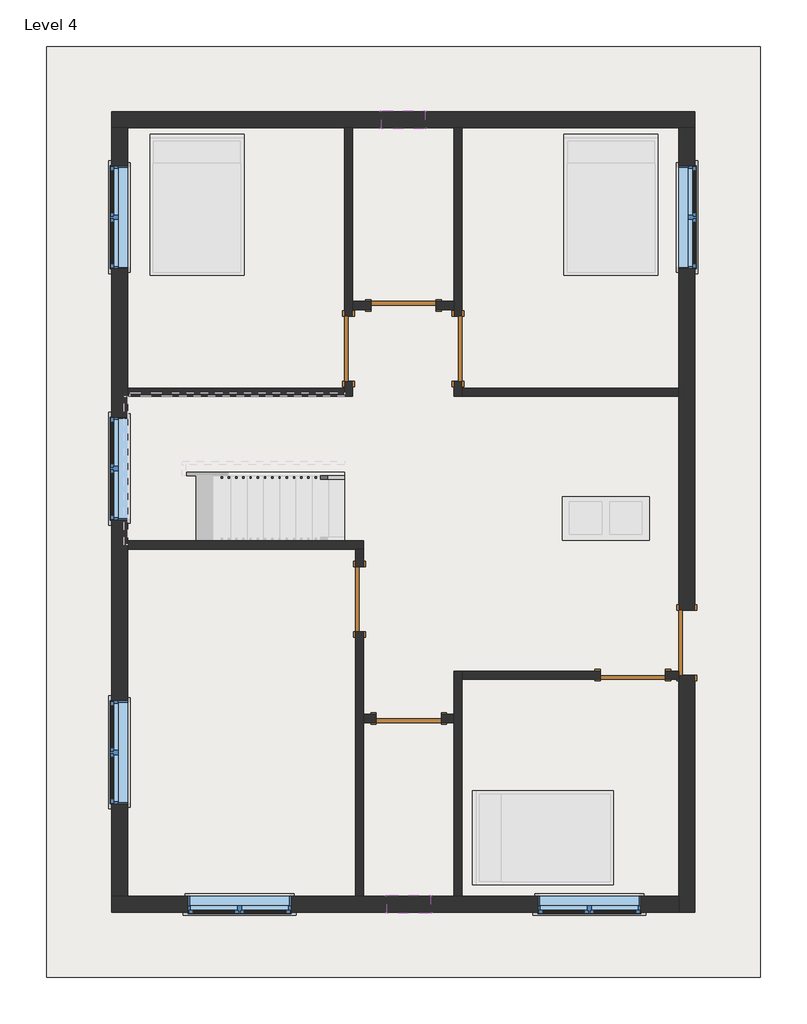
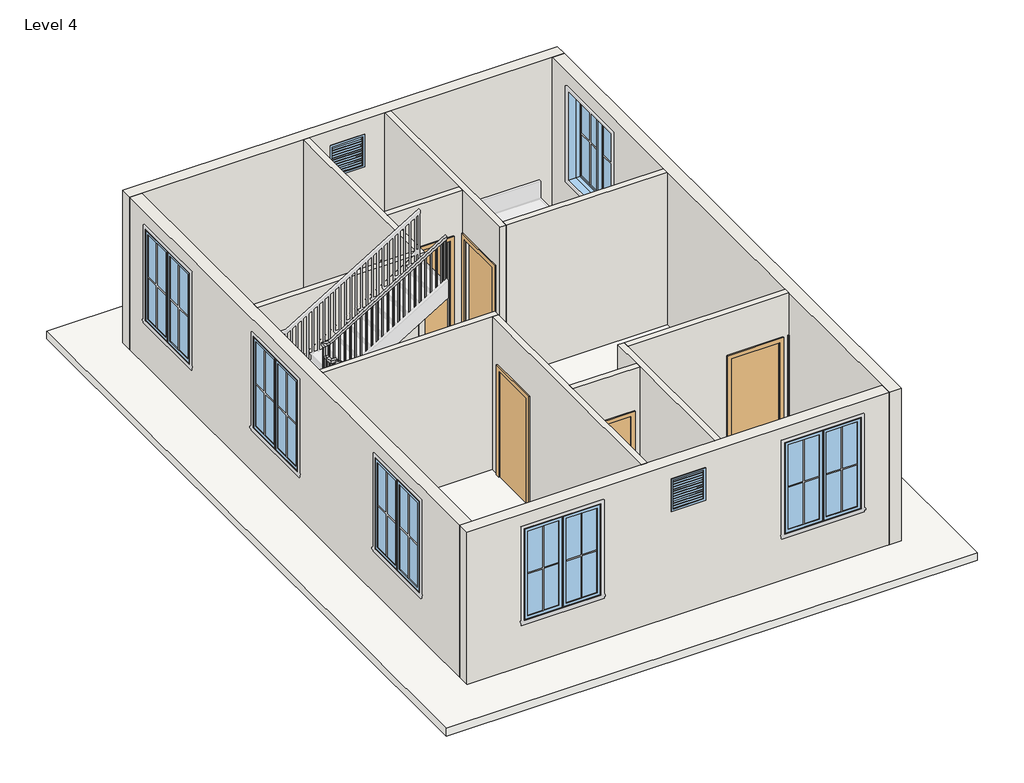
# One storey, part 1 of 2: 14 walls, 8 windows, 7 doors, 1 railing, 1 roof, 1 slab.
"""IFC4 building model written with IfcOpenShell, lengths in millimetres."""

from ifc_helpers import new_model, si_unit, frame, origin, place, context, project, spatial, polyline, outline, extrude, faceted_brep, transform, mapped, element, save
from components import door_305aa2a5, door_e5f9f3c4, door_0ca8825f, window_9ac97e1a, window_f2d8fef0

model = new_model("IFC4")

# Units and contexts
model_context = context("Model", 3, world=origin())
ifc_project = project(units=[si_unit("LENGTHUNIT", "METRE", prefix="MILLI")], contexts=[model_context])

# Site, building, storey
site = spatial("IfcSite", under=ifc_project)
building = spatial("IfcBuilding", under=site)
storey = spatial("IfcBuildingStorey", under=building, Name="Level 4", Elevation=6400.8)

# Doors
placement = place(None, origin())
door_shape = door_305aa2a5(model_context)
element("IfcDoor", 1, ObjectType="Single-Flush : 36\" x 84\"", at=placement, inside=storey, context=model_context, shape_type="MappedRepresentation", body=[
    mapped(door_shape, transform((-2023.6910855, 2116.5303617, 6400.8), x_axis=(0.0, -1.0, 0.0), y_axis=(1.0, 0.0, 0.0), z_axis=(0.0, 0.0, 1.0))),
])
element("IfcDoor", 2, ObjectType="Single-Flush : 36\" x 84\"", at=placement, inside=storey, context=model_context, shape_type="MappedRepresentation", body=[
    mapped(door_shape, transform((-1179.1410855, -3078.1725945, 6400.8), x_axis=(1.0, 0.0, 0.0), y_axis=(0.0, 1.0, 0.0), z_axis=(0.0, 0.0, 1.0))),
])
element("IfcDoor", 3, ObjectType="Single-Flush : 36\" x 84\"", at=placement, inside=storey, context=model_context, shape_type="MappedRepresentation", body=[
    mapped(door_shape, transform((1970.4589145, -2468.1696383, 6400.8), x_axis=(1.0, 0.0, 0.0), y_axis=(0.0, 1.0, 0.0), z_axis=(0.0, 0.0, 1.0))),
])
door_2_shape = door_e5f9f3c4(model_context)
element("IfcDoor", 4, ObjectType="Single-Flush : 36\" x 84\"", at=placement, inside=storey, context=model_context, shape_type="MappedRepresentation", body=[
    mapped(door_2_shape, transform((-486.9910855, 2116.5303617, 6400.8), x_axis=(0.0, -1.0, 0.0), y_axis=(1.0, 0.0, 0.0), z_axis=(0.0, 0.0, 1.0))),
])
element("IfcDoor", 5, ObjectType="Single-Flush : 36\" x 84\"", at=placement, inside=storey, context=model_context, shape_type="MappedRepresentation", body=[
    mapped(door_2_shape, transform((-1871.2910855, -1401.3696383, 6400.8), x_axis=(0.0, 1.0, 0.0), y_axis=(-1.0, 0.0, 0.0), z_axis=(0.0, 0.0, 1.0))),
])
element("IfcDoor", 6, ObjectType="Single-Flush : 36\" x 84\"", at=placement, inside=storey, context=model_context, shape_type="MappedRepresentation", body=[
    mapped(door_2_shape, transform((-1255.3410855, 2726.1303617, 6400.8), x_axis=(1.0, 0.0, 0.0), y_axis=(0.0, 1.0, 0.0), z_axis=(0.0, 0.0, 1.0))),
])
door_3_shape = door_0ca8825f(model_context)
element("IfcDoor", 7, ObjectType="Single-Flush : 36\" x 84\"", at=placement, inside=storey, context=model_context, shape_type="MappedRepresentation", body=[
    mapped(door_3_shape, transform((2732.4589145, -2010.9696383, 6400.8), x_axis=(0.0, 1.0, 0.0), y_axis=(-1.0, 0.0, 0.0), z_axis=(0.0, 0.0, 1.0))),
])

# Railing
element("IfcRailing", 8, ObjectType="Handrail - Rectangular", at=placement, inside=storey, context=model_context, shape_type="SolidModel", body=[
    faceted_brep([(-2080.8410855, 281.3803617, 7453.7454545), (-2080.8410855, 281.3803617, 7394.3439943), (-2080.8410855, 332.1803617, 7394.3439943), (-2080.8410855, 332.1803617, 7453.7454545), (-4290.6410855, 281.3803617, 8793.0181818), (-4341.4410855, 281.3803617, 8764.4046004), (-4341.4410855, 332.1803617, 8764.4046004), (-4290.6410855, 332.1803617, 8793.0181818), (-4290.6410855, 281.3803617, 8839.2), (-4341.4410855, 281.3803617, 8788.4), (-4341.4410855, 332.1803617, 8788.4), (-4290.6410855, 332.1803617, 8839.2), (-4417.6410855, 281.3803617, 8839.2), (-4417.6410855, 281.3803617, 8788.4), (-4366.8410855, 332.1803617, 8788.4), (-4366.8410855, 332.1803617, 8839.2), (-4417.6410855, 408.3803617, 8839.2), (-4417.6410855, 408.3803617, 8788.4), (-4366.8410855, 408.3803617, 8788.4), (-4366.8410855, 408.3803617, 8839.2), (-4417.6410855, 459.1803617, 8839.2), (-4417.6410855, 509.9803617, 8788.4), (-4366.8410855, 509.9803617, 8788.4), (-4366.8410855, 459.1803617, 8839.2), (-4417.6410855, 459.1803617, 9023.9272727), (-4417.6410855, 509.9803617, 8973.1272727), (-4366.8410855, 509.9803617, 8973.1272727), (-4366.8410855, 459.1803617, 9023.9272727), (-4417.6410855, 586.1803617, 9023.9272727), (-4417.6410855, 586.1803617, 8973.1272727), (-4366.8410855, 535.3803617, 8973.1272727), (-4366.8410855, 535.3803617, 9023.9272727), (-4290.6410855, 586.1803617, 9023.9272727), (-4276.4486761, 586.1803617, 8973.1272727), (-4276.4486761, 535.3803617, 8973.1272727), (-4290.6410855, 535.3803617, 9023.9272727), (-2080.8410855, 586.1803617, 10363.2), (-2080.8410855, 535.3803617, 10363.2), (-2080.8410855, 535.3803617, 10303.7985397), (-2080.8410855, 586.1803617, 10303.7985397)], [[[0, 1, 2, 3]], [[1, 0, 4, 5]], [[2, 1, 5, 6]], [[3, 2, 6, 7]], [[0, 3, 7, 4]], [[5, 4, 8, 9]], [[6, 5, 9, 10]], [[7, 6, 10, 11]], [[4, 7, 11, 8]], [[9, 8, 12, 13]], [[10, 9, 13, 14]], [[11, 10, 14, 15]], [[8, 11, 15, 12]], [[13, 12, 16, 17]], [[14, 13, 17, 18]], [[15, 14, 18, 19]], [[12, 15, 19, 16]], [[17, 16, 20, 21]], [[18, 17, 21, 22]], [[19, 18, 22, 23]], [[16, 19, 23, 20]], [[21, 20, 24, 25]], [[22, 21, 25, 26]], [[23, 22, 26, 27]], [[20, 23, 27, 24]], [[25, 24, 28, 29]], [[26, 25, 29, 30]], [[27, 26, 30, 31]], [[24, 27, 31, 28]], [[29, 28, 32, 33]], [[30, 29, 33, 34]], [[31, 30, 34, 35]], [[28, 31, 35, 32]], [[36, 37, 38, 39]], [[33, 32, 36, 39]], [[34, 33, 39, 38]], [[35, 34, 38, 37]], [[32, 35, 37, 36]]]),
    extrude(outline(polyline([(10263.3894488, -2147.5160855), (10251.8439943, -2166.5660855), (9310.2545455, -2166.5660855), (9310.2545455, -2147.5160855), (10263.3894488, -2147.5160855)])), frame((0.0, 551.2553617, 0.0), z_axis=(0.0, 1.0, 0.0), x_axis=(0.0, 0.0, 1.0)), (0.0, 0.0, 1.0), 19.05),
    extrude(outline(polyline([(10201.8136913, -2249.1160855), (10190.2682367, -2268.1660855), (9310.2545455, -2268.1660855), (9310.2545455, -2249.1160855), (10201.8136913, -2249.1160855)])), frame((0.0, 551.2553617, 0.0), z_axis=(0.0, 1.0, 0.0), x_axis=(0.0, 0.0, 1.0)), (0.0, 0.0, 1.0), 19.05),
    extrude(outline(polyline([(10140.2379337, -2350.7160855), (10128.6924791, -2369.7660855), (9171.7090909, -2369.7660855), (9171.7090909, -2350.7160855), (10140.2379337, -2350.7160855)])), frame((0.0, 551.2553617, 0.0), z_axis=(0.0, 1.0, 0.0), x_axis=(0.0, 0.0, 1.0)), (0.0, 0.0, 1.0), 19.05),
    extrude(outline(polyline([(10078.6621761, -2452.3160855), (10067.1167216, -2471.3660855), (9171.7090909, -2471.3660855), (9171.7090909, -2452.3160855), (10078.6621761, -2452.3160855)])), frame((0.0, 551.2553617, 0.0), z_axis=(0.0, 1.0, 0.0), x_axis=(0.0, 0.0, 1.0)), (0.0, 0.0, 1.0), 19.05),
    extrude(outline(polyline([(10017.0864185, -2553.9160855), (10005.540964, -2572.9660855), (9033.1636364, -2572.9660855), (9033.1636364, -2553.9160855), (10017.0864185, -2553.9160855)])), frame((0.0, 551.2553617, 0.0), z_axis=(0.0, 1.0, 0.0), x_axis=(0.0, 0.0, 1.0)), (0.0, 0.0, 1.0), 19.05),
    extrude(outline(polyline([(9955.510661, -2655.5160855), (9943.9652064, -2674.5660855), (9033.1636364, -2674.5660855), (9033.1636364, -2655.5160855), (9955.510661, -2655.5160855)])), frame((0.0, 551.2553617, 0.0), z_axis=(0.0, 1.0, 0.0), x_axis=(0.0, 0.0, 1.0)), (0.0, 0.0, 1.0), 19.05),
    extrude(outline(polyline([(9893.9349034, -2757.1160855), (9882.3894488, -2776.1660855), (9033.1636364, -2776.1660855), (9033.1636364, -2757.1160855), (9893.9349034, -2757.1160855)])), frame((0.0, 551.2553617, 0.0), z_axis=(0.0, 1.0, 0.0), x_axis=(0.0, 0.0, 1.0)), (0.0, 0.0, 1.0), 19.05),
    extrude(outline(polyline([(9832.3591458, -2858.7160855), (9820.8136913, -2877.7660855), (8894.6181818, -2877.7660855), (8894.6181818, -2858.7160855), (9832.3591458, -2858.7160855)])), frame((0.0, 551.2553617, 0.0), z_axis=(0.0, 1.0, 0.0), x_axis=(0.0, 0.0, 1.0)), (0.0, 0.0, 1.0), 19.05),
    extrude(outline(polyline([(9770.7833882, -2960.3160855), (9759.2379337, -2979.3660855), (8894.6181818, -2979.3660855), (8894.6181818, -2960.3160855), (9770.7833882, -2960.3160855)])), frame((0.0, 551.2553617, 0.0), z_axis=(0.0, 1.0, 0.0), x_axis=(0.0, 0.0, 1.0)), (0.0, 0.0, 1.0), 19.05),
    extrude(outline(polyline([(9709.2076307, -3061.9160855), (9697.6621761, -3080.9660855), (8756.0727273, -3080.9660855), (8756.0727273, -3061.9160855), (9709.2076307, -3061.9160855)])), frame((0.0, 551.2553617, 0.0), z_axis=(0.0, 1.0, 0.0), x_axis=(0.0, 0.0, 1.0)), (0.0, 0.0, 1.0), 19.05),
    extrude(outline(polyline([(9647.6318731, -3163.5160855), (9636.0864185, -3182.5660855), (8756.0727273, -3182.5660855), (8756.0727273, -3163.5160855), (9647.6318731, -3163.5160855)])), frame((0.0, 551.2553617, 0.0), z_axis=(0.0, 1.0, 0.0), x_axis=(0.0, 0.0, 1.0)), (0.0, 0.0, 1.0), 19.05),
    extrude(outline(polyline([(9586.0561155, -3265.1160855), (9574.510661, -3284.1660855), (8617.5272727, -3284.1660855), (8617.5272727, -3265.1160855), (9586.0561155, -3265.1160855)])), frame((0.0, 551.2553617, 0.0), z_axis=(0.0, 1.0, 0.0), x_axis=(0.0, 0.0, 1.0)), (0.0, 0.0, 1.0), 19.05),
    extrude(outline(polyline([(9524.4803579, -3366.7160855), (9512.9349034, -3385.7660855), (8617.5272727, -3385.7660855), (8617.5272727, -3366.7160855), (9524.4803579, -3366.7160855)])), frame((0.0, 551.2553617, 0.0), z_axis=(0.0, 1.0, 0.0), x_axis=(0.0, 0.0, 1.0)), (0.0, 0.0, 1.0), 19.05),
    extrude(outline(polyline([(9462.9046004, -3468.3160855), (9451.3591458, -3487.3660855), (8478.9818182, -3487.3660855), (8478.9818182, -3468.3160855), (9462.9046004, -3468.3160855)])), frame((0.0, 551.2553617, 0.0), z_axis=(0.0, 1.0, 0.0), x_axis=(0.0, 0.0, 1.0)), (0.0, 0.0, 1.0), 19.05),
    extrude(outline(polyline([(9401.3288428, -3569.9160855), (9389.7833882, -3588.9660855), (8478.9818182, -3588.9660855), (8478.9818182, -3569.9160855), (9401.3288428, -3569.9160855)])), frame((0.0, 551.2553617, 0.0), z_axis=(0.0, 1.0, 0.0), x_axis=(0.0, 0.0, 1.0)), (0.0, 0.0, 1.0), 19.05),
    extrude(outline(polyline([(9339.7530852, -3671.5160855), (9328.2076307, -3690.5660855), (8478.9818182, -3690.5660855), (8478.9818182, -3671.5160855), (9339.7530852, -3671.5160855)])), frame((0.0, 551.2553617, 0.0), z_axis=(0.0, 1.0, 0.0), x_axis=(0.0, 0.0, 1.0)), (0.0, 0.0, 1.0), 19.05),
    extrude(outline(polyline([(9278.1773276, -3773.1160855), (9266.6318731, -3792.1660855), (8340.4363636, -3792.1660855), (8340.4363636, -3773.1160855), (9278.1773276, -3773.1160855)])), frame((0.0, 551.2553617, 0.0), z_axis=(0.0, 1.0, 0.0), x_axis=(0.0, 0.0, 1.0)), (0.0, 0.0, 1.0), 19.05),
    extrude(outline(polyline([(9216.60157, -3874.7160855), (9205.0561155, -3893.7660855), (8340.4363636, -3893.7660855), (8340.4363636, -3874.7160855), (9216.60157, -3874.7160855)])), frame((0.0, 551.2553617, 0.0), z_axis=(0.0, 1.0, 0.0), x_axis=(0.0, 0.0, 1.0)), (0.0, 0.0, 1.0), 19.05),
    extrude(outline(polyline([(9155.0258125, -3976.3160855), (9143.4803579, -3995.3660855), (8201.8909091, -3995.3660855), (8201.8909091, -3976.3160855), (9155.0258125, -3976.3160855)])), frame((0.0, 551.2553617, 0.0), z_axis=(0.0, 1.0, 0.0), x_axis=(0.0, 0.0, 1.0)), (0.0, 0.0, 1.0), 19.05),
    extrude(outline(polyline([(9093.4500549, -4077.9160855), (9081.9046004, -4096.9660855), (8201.8909091, -4096.9660855), (8201.8909091, -4077.9160855), (9093.4500549, -4077.9160855)])), frame((0.0, 551.2553617, 0.0), z_axis=(0.0, 1.0, 0.0), x_axis=(0.0, 0.0, 1.0)), (0.0, 0.0, 1.0), 19.05),
    extrude(outline(polyline([(9031.8742973, -4179.5160855), (9020.3288428, -4198.5660855), (8063.3454545, -4198.5660855), (8063.3454545, -4179.5160855), (9031.8742973, -4179.5160855)])), frame((0.0, 551.2553617, 0.0), z_axis=(0.0, 1.0, 0.0), x_axis=(0.0, 0.0, 1.0)), (0.0, 0.0, 1.0), 19.05),
    extrude(outline(polyline([(8970.2985397, -4281.1160855), (8958.7530852, -4300.1660855), (8063.3454545, -4300.1660855), (8063.3454545, -4281.1160855), (8970.2985397, -4281.1160855)])), frame((0.0, 551.2553617, 0.0), z_axis=(0.0, 1.0, 0.0), x_axis=(0.0, 0.0, 1.0)), (0.0, 0.0, 1.0), 19.05),
    extrude(outline(polyline([(-4382.7160855, 500.4553617), (-4401.7660855, 500.4553617), (-4401.7660855, 519.5053617), (-4382.7160855, 519.5053617), (-4382.7160855, 500.4553617)])), frame((0.0, 0.0, 7924.8), z_axis=(0.0, 0.0, 1.0), x_axis=(1.0, 0.0, 0.0)), (0.0, 0.0, 1.0), 1048.3272727),
    extrude(outline(polyline([(-4382.7160855, 398.8553617), (-4401.7660855, 398.8553617), (-4401.7660855, 417.9053617), (-4382.7160855, 417.9053617), (-4382.7160855, 398.8553617)])), frame((0.0, 0.0, 7924.8), z_axis=(0.0, 0.0, 1.0), x_axis=(1.0, 0.0, 0.0)), (0.0, 0.0, 1.0), 863.6),
    extrude(outline(polyline([(-4306.5160855, 316.3053617), (-4306.5160855, 297.2553617), (-4325.5660855, 297.2553617), (-4325.5660855, 316.3053617), (-4306.5160855, 316.3053617)])), frame((0.0, 0.0, 7786.2545455), z_axis=(0.0, 0.0, 1.0), x_axis=(1.0, 0.0, 0.0)), (0.0, 0.0, 1.0), 1002.1454545),
    extrude(outline(polyline([(8681.6621761, -4204.9160855), (8693.2076307, -4223.9660855), (7786.2545455, -4223.9660855), (7786.2545455, -4204.9160855), (8681.6621761, -4204.9160855)])), frame((0.0, 297.2553617, 0.0), z_axis=(0.0, 1.0, 0.0), x_axis=(0.0, 0.0, 1.0)), (0.0, 0.0, 1.0), 19.05),
    extrude(outline(polyline([(8620.0864185, -4103.3160855), (8631.6318731, -4122.3660855), (7647.7090909, -4122.3660855), (7647.7090909, -4103.3160855), (8620.0864185, -4103.3160855)])), frame((0.0, 297.2553617, 0.0), z_axis=(0.0, 1.0, 0.0), x_axis=(0.0, 0.0, 1.0)), (0.0, 0.0, 1.0), 19.05),
    extrude(outline(polyline([(8558.510661, -4001.7160855), (8570.0561155, -4020.7660855), (7647.7090909, -4020.7660855), (7647.7090909, -4001.7160855), (8558.510661, -4001.7160855)])), frame((0.0, 297.2553617, 0.0), z_axis=(0.0, 1.0, 0.0), x_axis=(0.0, 0.0, 1.0)), (0.0, 0.0, 1.0), 19.05),
    extrude(outline(polyline([(8496.9349034, -3900.1160855), (8508.4803579, -3919.1660855), (7647.7090909, -3919.1660855), (7647.7090909, -3900.1160855), (8496.9349034, -3900.1160855)])), frame((0.0, 297.2553617, 0.0), z_axis=(0.0, 1.0, 0.0), x_axis=(0.0, 0.0, 1.0)), (0.0, 0.0, 1.0), 19.05),
    extrude(outline(polyline([(8435.3591458, -3798.5160855), (8446.9046004, -3817.5660855), (7509.1636364, -3817.5660855), (7509.1636364, -3798.5160855), (8435.3591458, -3798.5160855)])), frame((0.0, 297.2553617, 0.0), z_axis=(0.0, 1.0, 0.0), x_axis=(0.0, 0.0, 1.0)), (0.0, 0.0, 1.0), 19.05),
    extrude(outline(polyline([(8373.7833882, -3696.9160855), (8385.3288428, -3715.9660855), (7509.1636364, -3715.9660855), (7509.1636364, -3696.9160855), (8373.7833882, -3696.9160855)])), frame((0.0, 297.2553617, 0.0), z_axis=(0.0, 1.0, 0.0), x_axis=(0.0, 0.0, 1.0)), (0.0, 0.0, 1.0), 19.05),
    extrude(outline(polyline([(8312.2076307, -3595.3160855), (8323.7530852, -3614.3660855), (7370.6181818, -3614.3660855), (7370.6181818, -3595.3160855), (8312.2076307, -3595.3160855)])), frame((0.0, 297.2553617, 0.0), z_axis=(0.0, 1.0, 0.0), x_axis=(0.0, 0.0, 1.0)), (0.0, 0.0, 1.0), 19.05),
    extrude(outline(polyline([(8250.6318731, -3493.7160855), (8262.1773276, -3512.7660855), (7370.6181818, -3512.7660855), (7370.6181818, -3493.7160855), (8250.6318731, -3493.7160855)])), frame((0.0, 297.2553617, 0.0), z_axis=(0.0, 1.0, 0.0), x_axis=(0.0, 0.0, 1.0)), (0.0, 0.0, 1.0), 19.05),
    extrude(outline(polyline([(8189.0561155, -3392.1160855), (8200.60157, -3411.1660855), (7232.0727273, -3411.1660855), (7232.0727273, -3392.1160855), (8189.0561155, -3392.1160855)])), frame((0.0, 297.2553617, 0.0), z_axis=(0.0, 1.0, 0.0), x_axis=(0.0, 0.0, 1.0)), (0.0, 0.0, 1.0), 19.05),
    extrude(outline(polyline([(8127.4803579, -3290.5160855), (8139.0258125, -3309.5660855), (7232.0727273, -3309.5660855), (7232.0727273, -3290.5160855), (8127.4803579, -3290.5160855)])), frame((0.0, 297.2553617, 0.0), z_axis=(0.0, 1.0, 0.0), x_axis=(0.0, 0.0, 1.0)), (0.0, 0.0, 1.0), 19.05),
    extrude(outline(polyline([(8065.9046004, -3188.9160855), (8077.4500549, -3207.9660855), (7093.5272727, -3207.9660855), (7093.5272727, -3188.9160855), (8065.9046004, -3188.9160855)])), frame((0.0, 297.2553617, 0.0), z_axis=(0.0, 1.0, 0.0), x_axis=(0.0, 0.0, 1.0)), (0.0, 0.0, 1.0), 19.05),
    extrude(outline(polyline([(8004.3288428, -3087.3160855), (8015.8742973, -3106.3660855), (7093.5272727, -3106.3660855), (7093.5272727, -3087.3160855), (8004.3288428, -3087.3160855)])), frame((0.0, 297.2553617, 0.0), z_axis=(0.0, 1.0, 0.0), x_axis=(0.0, 0.0, 1.0)), (0.0, 0.0, 1.0), 19.05),
    extrude(outline(polyline([(7942.7530852, -2985.7160855), (7954.2985397, -3004.7660855), (7093.5272727, -3004.7660855), (7093.5272727, -2985.7160855), (7942.7530852, -2985.7160855)])), frame((0.0, 297.2553617, 0.0), z_axis=(0.0, 1.0, 0.0), x_axis=(0.0, 0.0, 1.0)), (0.0, 0.0, 1.0), 19.05),
    extrude(outline(polyline([(7881.1773276, -2884.1160855), (7892.7227822, -2903.1660855), (6954.9818182, -2903.1660855), (6954.9818182, -2884.1160855), (7881.1773276, -2884.1160855)])), frame((0.0, 297.2553617, 0.0), z_axis=(0.0, 1.0, 0.0), x_axis=(0.0, 0.0, 1.0)), (0.0, 0.0, 1.0), 19.05),
    extrude(outline(polyline([(7819.60157, -2782.5160855), (7831.1470246, -2801.5660855), (6954.9818182, -2801.5660855), (6954.9818182, -2782.5160855), (7819.60157, -2782.5160855)])), frame((0.0, 297.2553617, 0.0), z_axis=(0.0, 1.0, 0.0), x_axis=(0.0, 0.0, 1.0)), (0.0, 0.0, 1.0), 19.05),
    extrude(outline(polyline([(7758.0258125, -2680.9160855), (7769.571267, -2699.9660855), (6816.4363636, -2699.9660855), (6816.4363636, -2680.9160855), (7758.0258125, -2680.9160855)])), frame((0.0, 297.2553617, 0.0), z_axis=(0.0, 1.0, 0.0), x_axis=(0.0, 0.0, 1.0)), (0.0, 0.0, 1.0), 19.05),
    extrude(outline(polyline([(7696.4500549, -2579.3160855), (7707.9955094, -2598.3660855), (6816.4363636, -2598.3660855), (6816.4363636, -2579.3160855), (7696.4500549, -2579.3160855)])), frame((0.0, 297.2553617, 0.0), z_axis=(0.0, 1.0, 0.0), x_axis=(0.0, 0.0, 1.0)), (0.0, 0.0, 1.0), 19.05),
    extrude(outline(polyline([(7634.8742973, -2477.7160855), (7646.4197519, -2496.7660855), (6677.8909091, -2496.7660855), (6677.8909091, -2477.7160855), (7634.8742973, -2477.7160855)])), frame((0.0, 297.2553617, 0.0), z_axis=(0.0, 1.0, 0.0), x_axis=(0.0, 0.0, 1.0)), (0.0, 0.0, 1.0), 19.05),
    extrude(outline(polyline([(7573.2985397, -2376.1160855), (7584.8439943, -2395.1660855), (6677.8909091, -2395.1660855), (6677.8909091, -2376.1160855), (7573.2985397, -2376.1160855)])), frame((0.0, 297.2553617, 0.0), z_axis=(0.0, 1.0, 0.0), x_axis=(0.0, 0.0, 1.0)), (0.0, 0.0, 1.0), 19.05),
    extrude(outline(polyline([(7511.7227822, -2274.5160855), (7523.2682367, -2293.5660855), (6539.3454545, -2293.5660855), (6539.3454545, -2274.5160855), (7511.7227822, -2274.5160855)])), frame((0.0, 297.2553617, 0.0), z_axis=(0.0, 1.0, 0.0), x_axis=(0.0, 0.0, 1.0)), (0.0, 0.0, 1.0), 19.05),
    extrude(outline(polyline([(7450.1470246, -2172.9160855), (7461.6924791, -2191.9660855), (6539.3454545, -2191.9660855), (6539.3454545, -2172.9160855), (7450.1470246, -2172.9160855)])), frame((0.0, 297.2553617, 0.0), z_axis=(0.0, 1.0, 0.0), x_axis=(0.0, 0.0, 1.0)), (0.0, 0.0, 1.0), 19.05),
    extrude(outline(polyline([(-4382.7160855, 551.2553617), (-4401.7660855, 551.2553617), (-4401.7660855, 570.3053617), (-4382.7160855, 570.3053617), (-4382.7160855, 551.2553617)])), frame((0.0, 0.0, 7924.8), z_axis=(0.0, 0.0, 1.0), x_axis=(1.0, 0.0, 0.0)), (0.0, 0.0, 1.0), 1048.3272727),
    extrude(outline(polyline([(-4382.7160855, 316.3053617), (-4382.7160855, 297.2553617), (-4401.7660855, 297.2553617), (-4401.7660855, 316.3053617), (-4382.7160855, 316.3053617)])), frame((0.0, 0.0, 7924.8), z_axis=(0.0, 0.0, 1.0), x_axis=(1.0, 0.0, 0.0)), (0.0, 0.0, 1.0), 863.6),
    extrude(outline(polyline([(10303.7985397, -2080.8410855), (10292.2530852, -2099.8910855), (9310.2545455, -2099.8910855), (9310.2545455, -2080.8410855), (10303.7985397, -2080.8410855)])), frame((0.0, 551.2553617, 0.0), z_axis=(0.0, 1.0, 0.0), x_axis=(0.0, 0.0, 1.0)), (0.0, 0.0, 1.0), 19.05),
    extrude(outline(polyline([(7394.3439943, -2080.8410855), (7405.8894488, -2099.8910855), (6539.3454545, -2099.8910855), (6539.3454545, -2080.8410855), (7394.3439943, -2080.8410855)])), frame((0.0, 297.2553617, 0.0), z_axis=(0.0, 1.0, 0.0), x_axis=(0.0, 0.0, 1.0)), (0.0, 0.0, 1.0), 19.05),
])

# Roof
element("IfcRoof", 9, ObjectType="ROOF 6\"", at=placement, inside=storey, context=model_context, shape_type="SweptSolid", body=[
    extrude(outline(polyline([(-6271.8410855, 6364.6803617), (3761.1589145, 6364.6803617), (3761.1589145, -6716.3196383), (-6271.8410855, -6716.3196383), (-6271.8410855, 6364.6803617)])), frame((0.0, 0.0, 6248.4), z_axis=(0.0, 0.0, 1.0), x_axis=(1.0, 0.0, 0.0)), (0.0, 0.0, 1.0), 152.4),
])

# Slab
element("IfcSlab", 10, ObjectType="FLOOR 6\"", at=placement, inside=storey, context=model_context, shape_type="SweptSolid", body=[
    extrude(outline(polyline([(2846.7589145, 5450.2803617), (2846.7589145, -5801.9196383), (-5357.4410855, -5801.9196383), (-5357.4410855, 5450.2803617), (2846.7589145, 5450.2803617)])), frame((0.0, 0.0, 6248.4), z_axis=(0.0, 0.0, 1.0), x_axis=(1.0, 0.0, 0.0)), (0.0, 0.0, 1.0), 152.4),
])

# Walls
element("IfcWall", 11, ObjectType="WALL 4.5\"", at=placement, inside=storey, context=model_context, shape_type="Brep", body=[
    faceted_brep([(-2080.8410855, 1659.3303617, 8534.4), (-2080.8410855, 1659.3303617, 6400.8), (-2080.8410855, 1564.0803617, 6400.8), (-2080.8410855, 1449.7803617, 6400.8), (-2080.8410855, 1449.7803617, 9448.8), (-2080.8410855, 1564.0803617, 9448.8), (-2080.8410855, 5221.6803617, 9448.8), (-2080.8410855, 5221.6803617, 6400.8), (-2080.8410855, 2573.7303617, 6400.8), (-2080.8410855, 2573.7303617, 8534.4), (-1966.5410855, 1449.7803617, 6400.8), (-1966.5410855, 1659.3303617, 6400.8), (-1966.5410855, 1659.3303617, 8534.4), (-1966.5410855, 2573.7303617, 8534.4), (-1966.5410855, 2573.7303617, 6400.8), (-1966.5410855, 2668.9803617, 6400.8), (-1966.5410855, 2783.2803617, 6400.8), (-1966.5410855, 5221.6803617, 6400.8), (-1966.5410855, 5221.6803617, 9448.8), (-1966.5410855, 2783.2803617, 9448.8), (-1966.5410855, 2668.9803617, 9448.8), (-1966.5410855, 1449.7803617, 9448.8)], [[[0, 1, 2, 3, 4, 5, 6, 7, 8, 9]], [[10, 11, 12, 13, 14, 15, 16, 17, 18, 19, 20, 21]], [[8, 7, 17, 16, 15, 14]], [[3, 2, 1, 11, 10]], [[7, 6, 18, 17]], [[4, 3, 10, 21]], [[12, 11, 1, 0]], [[13, 12, 0, 9]], [[14, 13, 9, 8]], [[6, 5, 4, 21, 20, 19, 18]]]),
])
element("IfcWall", 12, ObjectType="WALL 4.5\"", at=placement, inside=storey, context=model_context, shape_type="SweptSolid", body=[
    extrude(outline(polyline([(-5128.8410855, 1564.0803617), (-2080.8410855, 1564.0803617), (-2080.8410855, 1449.7803617), (-5128.8410855, 1449.7803617), (-5128.8410855, 1564.0803617)])), frame((0.0, 0.0, 6400.8), z_axis=(0.0, 0.0, 1.0), x_axis=(1.0, 0.0, 0.0)), (0.0, 0.0, 1.0), 3048.0),
])
element("IfcWall", 13, ObjectType="WALL 4.5\"", at=placement, inside=storey, context=model_context, shape_type="Brep", body=[
    faceted_brep([(-544.1410855, 1659.3303617, 8534.4), (-544.1410855, 1659.3303617, 6400.8), (-544.1410855, 1449.7803617, 6400.8), (-544.1410855, 1449.7803617, 9448.8), (-544.1410855, 2668.9803617, 9448.8), (-544.1410855, 2783.2803617, 9448.8), (-544.1410855, 5221.6803617, 9448.8), (-544.1410855, 5221.6803617, 6400.8), (-544.1410855, 2783.2803617, 6400.8), (-544.1410855, 2668.9803617, 6400.8), (-544.1410855, 2573.7303617, 6400.8), (-544.1410855, 2573.7303617, 8534.4), (-429.8410855, 1449.7803617, 6400.8), (-429.8410855, 1564.0803617, 6400.8), (-429.8410855, 1659.3303617, 6400.8), (-429.8410855, 1659.3303617, 8534.4), (-429.8410855, 2573.7303617, 8534.4), (-429.8410855, 2573.7303617, 6400.8), (-429.8410855, 5221.6803617, 6400.8), (-429.8410855, 5221.6803617, 9448.8), (-429.8410855, 1564.0803617, 9448.8), (-429.8410855, 1449.7803617, 9448.8)], [[[0, 1, 2, 3, 4, 5, 6, 7, 8, 9, 10, 11]], [[12, 13, 14, 15, 16, 17, 18, 19, 20, 21]], [[2, 1, 14, 13, 12]], [[10, 9, 8, 7, 18, 17]], [[7, 6, 19, 18]], [[3, 2, 12, 21]], [[15, 14, 1, 0]], [[16, 15, 0, 11]], [[17, 16, 11, 10]], [[6, 5, 4, 3, 21, 20, 19]]]),
])
element("IfcWall", 14, ObjectType="WALL 4.5\"", at=placement, inside=storey, context=model_context, shape_type="SweptSolid", body=[
    extrude(outline(polyline([(2618.1589145, 1449.7803617), (-429.8410855, 1449.7803617), (-429.8410855, 1564.0803617), (2618.1589145, 1564.0803617), (2618.1589145, 1449.7803617)])), frame((0.0, 0.0, 6400.8), z_axis=(0.0, 0.0, 1.0), x_axis=(1.0, 0.0, 0.0)), (0.0, 0.0, 1.0), 3048.0),
])
element("IfcWall", 15, ObjectType="WALL 4.5\"", at=placement, inside=storey, context=model_context, shape_type="Brep", body=[
    faceted_brep([(-5128.8410855, -696.5196383, 6400.8), (-1928.4410855, -696.5196383, 6400.8), (-1814.1410855, -696.5196383, 6400.8), (-1814.1410855, -696.5196383, 9448.8), (-1928.4410855, -696.5196383, 9448.8), (-5128.8410855, -696.5196383, 9448.8), (-5128.8410855, -582.2196383, 6400.8), (-5128.8410855, -582.2196383, 9448.8), (-1814.1410855, -582.2196383, 9448.8), (-1814.1410855, -582.2196383, 6400.8)], [[[0, 1, 2, 3, 4, 5]], [[6, 7, 8, 9]], [[2, 1, 0, 6, 9]], [[0, 5, 7, 6]], [[3, 2, 9, 8]], [[5, 4, 3, 8, 7]]]),
])
element("IfcWall", 16, ObjectType="WALL 4.5\"", at=placement, inside=storey, context=model_context, shape_type="Brep", body=[
    faceted_brep([(-1814.1410855, -944.1696383, 8534.4), (-1814.1410855, -944.1696383, 6400.8), (-1814.1410855, -696.5196383, 6400.8), (-1814.1410855, -696.5196383, 9448.8), (-1814.1410855, -3021.0225945, 9448.8), (-1814.1410855, -3135.3225945, 9448.8), (-1814.1410855, -5573.3196383, 9448.8), (-1814.1410855, -5573.3196383, 6400.8), (-1814.1410855, -3135.3225945, 6400.8), (-1814.1410855, -3021.0225945, 6400.8), (-1814.1410855, -1858.5696383, 6400.8), (-1814.1410855, -1858.5696383, 8534.4), (-1928.4410855, -696.5196383, 6400.8), (-1928.4410855, -944.1696383, 6400.8), (-1928.4410855, -944.1696383, 8534.4), (-1928.4410855, -1858.5696383, 8534.4), (-1928.4410855, -1858.5696383, 6400.8), (-1928.4410855, -5573.3196383, 6400.8), (-1928.4410855, -5573.3196383, 9448.8), (-1928.4410855, -696.5196383, 9448.8)], [[[0, 1, 2, 3, 4, 5, 6, 7, 8, 9, 10, 11]], [[12, 13, 14, 15, 16, 17, 18, 19]], [[2, 1, 13, 12]], [[10, 9, 8, 7, 17, 16]], [[3, 2, 12, 19]], [[7, 6, 18, 17]], [[14, 13, 1, 0]], [[15, 14, 0, 11]], [[16, 15, 11, 10]], [[6, 5, 4, 3, 19, 18]]]),
])
element("IfcWall", 17, ObjectType="WALL 4.5\"", at=placement, inside=storey, context=model_context, shape_type="SweptSolid", body=[
    extrude(outline(polyline([(8534.4, -721.9410855), (6400.8, -721.9410855), (6400.8, -544.1410855), (9448.8, -544.1410855), (9448.8, -1814.1410855), (6400.8, -1814.1410855), (6400.8, -1636.3410855), (8534.4, -1636.3410855), (8534.4, -721.9410855)])), frame((0.0, -3135.3225945, 0.0), z_axis=(0.0, 1.0, 0.0), x_axis=(0.0, 0.0, 1.0)), (0.0, 0.0, 1.0), 114.3),
])
element("IfcWall", 18, ObjectType="WALL 4.5\"", at=placement, inside=storey, context=model_context, shape_type="Brep", body=[
    faceted_brep([(-544.1410855, -2411.0196383, 6400.8), (-544.1410855, -3021.0225945, 6400.8), (-544.1410855, -3135.3225945, 6400.8), (-544.1410855, -5573.3196383, 6400.8), (-544.1410855, -5573.3196383, 9448.8), (-544.1410855, -3135.3225945, 9448.8), (-544.1410855, -3021.0225945, 9448.8), (-544.1410855, -2411.0196383, 9448.8), (-429.8410855, -2411.0196383, 6400.8), (-429.8410855, -2411.0196383, 9448.8), (-429.8410855, -2525.3196383, 9448.8), (-429.8410855, -5573.3196383, 9448.8), (-429.8410855, -5573.3196383, 6400.8), (-429.8410855, -2525.3196383, 6400.8)], [[[0, 1, 2, 3, 4, 5, 6, 7]], [[8, 9, 10, 11, 12, 13]], [[3, 2, 1, 0, 8, 13, 12]], [[4, 3, 12, 11]], [[0, 7, 9, 8]], [[7, 6, 5, 4, 11, 10, 9]]]),
])
element("IfcWall", 19, ObjectType="WALL 4.5\"", at=placement, inside=storey, context=model_context, shape_type="Brep", body=[
    faceted_brep([(2427.6589145, -2525.3196383, 8534.4), (2427.6589145, -2525.3196383, 6400.8), (2618.1589145, -2525.3196383, 6400.8), (2618.1589145, -2525.3196383, 9448.8), (-429.8410855, -2525.3196383, 9448.8), (-429.8410855, -2525.3196383, 6400.8), (1513.2589145, -2525.3196383, 6400.8), (1513.2589145, -2525.3196383, 8534.4), (2618.1589145, -2411.0196383, 6400.8), (2427.6589145, -2411.0196383, 6400.8), (2427.6589145, -2411.0196383, 8534.4), (1513.2589145, -2411.0196383, 8534.4), (1513.2589145, -2411.0196383, 6400.8), (-429.8410855, -2411.0196383, 6400.8), (-429.8410855, -2411.0196383, 9448.8), (2618.1589145, -2411.0196383, 9448.8), (2618.1589145, -2468.1696383, 6400.8)], [[[0, 1, 2, 3, 4, 5, 6, 7]], [[8, 9, 10, 11, 12, 13, 14, 15]], [[6, 5, 13, 12]], [[2, 1, 9, 8, 16]], [[5, 4, 14, 13]], [[3, 2, 16, 8, 15]], [[10, 9, 1, 0]], [[11, 10, 0, 7]], [[12, 11, 7, 6]], [[4, 3, 15, 14]]]),
])
element("IfcWall", 20, ObjectType="WALL 4.5\"", at=placement, inside=storey, context=model_context, shape_type="SweptSolid", body=[
    extrude(outline(polyline([(8534.4, -798.1410855), (6400.8, -798.1410855), (6400.8, -544.1410855), (9448.8, -544.1410855), (9448.8, -1966.5410855), (6400.8, -1966.5410855), (6400.8, -1712.5410855), (8534.4, -1712.5410855), (8534.4, -798.1410855)])), frame((0.0, 2668.9803617, 0.0), z_axis=(0.0, 1.0, 0.0), x_axis=(0.0, 0.0, 1.0)), (0.0, 0.0, 1.0), 114.3),
])
element("IfcWall", 21, ObjectType="WALL 9\"", at=placement, inside=storey, context=model_context, shape_type="Brep", body=[
    faceted_brep([(-5357.4410855, 5221.6803617, 6400.8), (-5128.8410855, 5221.6803617, 6400.8), (-2080.8410855, 5221.6803617, 6400.8), (-1966.5410855, 5221.6803617, 6400.8), (-544.1410855, 5221.6803617, 6400.8), (-429.8410855, 5221.6803617, 6400.8), (2618.1589145, 5221.6803617, 6400.8), (2846.7589145, 5221.6803617, 6400.8), (2846.7589145, 5221.6803617, 9448.8), (2618.1589145, 5221.6803617, 9448.8), (-429.8410855, 5221.6803617, 9448.8), (-544.1410855, 5221.6803617, 9448.8), (-1966.5410855, 5221.6803617, 9448.8), (-2080.8410855, 5221.6803617, 9448.8), (-5128.8410855, 5221.6803617, 9448.8), (-5357.4410855, 5221.6803617, 9448.8), (-950.5410855, 5221.6803617, 9144.0), (-950.5410855, 5221.6803617, 8534.4), (-1560.1410855, 5221.6803617, 8534.4), (-1560.1410855, 5221.6803617, 9144.0), (-5357.4410855, 5450.2803617, 6400.8), (-5357.4410855, 5450.2803617, 9448.8), (2846.7589145, 5450.2803617, 9448.8), (2846.7589145, 5450.2803617, 6400.8), (-950.5410855, 5450.2803617, 9144.0), (-1560.1410855, 5450.2803617, 9144.0), (-1560.1410855, 5450.2803617, 8534.4), (-950.5410855, 5450.2803617, 8534.4)], [[[0, 1, 2, 3, 4, 5, 6, 7, 8, 9, 10, 11, 12, 13, 14, 15], [16, 17, 18, 19]], [[20, 21, 22, 23], [24, 25, 26, 27]], [[7, 6, 5, 4, 3, 2, 1, 0, 20, 23]], [[8, 7, 23, 22]], [[0, 15, 21, 20]], [[17, 16, 24, 27]], [[18, 17, 27, 26]], [[19, 18, 26, 25]], [[16, 19, 25, 24]], [[15, 14, 13, 12, 11, 10, 9, 8, 22, 21]]]),
])
element("IfcWall", 22, ObjectType="WALL 9\"", at=placement, inside=storey, context=model_context, shape_type="Brep", body=[
    faceted_brep([(2618.1589145, 5221.6803617, 6400.8), (2618.1589145, 1564.0803617, 6400.8), (2618.1589145, 1449.7803617, 6400.8), (2618.1589145, -1553.7696383, 6400.8), (2618.1589145, -1553.7696383, 8534.4), (2618.1589145, -2468.1696383, 8534.4), (2618.1589145, -2468.1696383, 6400.8), (2618.1589145, -2525.3196383, 6400.8), (2618.1589145, -5573.3196383, 6400.8), (2618.1589145, -5801.9196383, 6400.8), (2618.1589145, -5801.9196383, 9448.8), (2618.1589145, -5573.3196383, 9448.8), (2618.1589145, -2525.3196383, 9448.8), (2618.1589145, -2411.0196383, 9448.8), (2618.1589145, 1449.7803617, 9448.8), (2618.1589145, 1564.0803617, 9448.8), (2618.1589145, 5221.6803617, 9448.8), (2618.1589145, 3240.4803617, 9144.0), (2618.1589145, 3240.4803617, 7315.2), (2618.1589145, 4688.2803617, 7315.2), (2618.1589145, 4688.2803617, 9144.0), (2846.7589145, -1553.7696383, 8534.4), (2846.7589145, -1553.7696383, 6400.8), (2846.7589145, 5221.6803617, 6400.8), (2846.7589145, 5221.6803617, 9448.8), (2846.7589145, -5801.9196383, 9448.8), (2846.7589145, -5801.9196383, 6400.8), (2846.7589145, -2468.1696383, 6400.8), (2846.7589145, -2468.1696383, 8534.4), (2846.7589145, 3240.4803617, 9144.0), (2846.7589145, 4688.2803617, 9144.0), (2846.7589145, 4688.2803617, 7315.2), (2846.7589145, 3240.4803617, 7315.2)], [[[0, 1, 2, 3, 4, 5, 6, 7, 8, 9, 10, 11, 12, 13, 14, 15, 16], [17, 18, 19, 20]], [[21, 22, 23, 24, 25, 26, 27, 28], [29, 30, 31, 32]], [[27, 26, 9, 8, 7, 6]], [[23, 22, 3, 2, 1, 0]], [[0, 16, 24, 23]], [[10, 9, 26, 25]], [[18, 17, 29, 32]], [[19, 18, 32, 31]], [[20, 19, 31, 30]], [[17, 20, 30, 29]], [[4, 3, 22, 21]], [[5, 4, 21, 28]], [[6, 5, 28, 27]], [[16, 15, 14, 13, 12, 11, 10, 25, 24]]]),
])
element("IfcWall", 23, ObjectType="WALL 9\"", at=placement, inside=storey, context=model_context, shape_type="Brep", body=[
    faceted_brep([(2618.1589145, -5573.3196383, 6400.8), (-429.8410855, -5573.3196383, 6400.8), (-544.1410855, -5573.3196383, 6400.8), (-1814.1410855, -5573.3196383, 6400.8), (-1928.4410855, -5573.3196383, 6400.8), (-5128.8410855, -5573.3196383, 6400.8), (-5357.4410855, -5573.3196383, 6400.8), (-5357.4410855, -5573.3196383, 9448.8), (-5128.8410855, -5573.3196383, 9448.8), (-1928.4410855, -5573.3196383, 9448.8), (-1814.1410855, -5573.3196383, 9448.8), (-544.1410855, -5573.3196383, 9448.8), (-429.8410855, -5573.3196383, 9448.8), (2618.1589145, -5573.3196383, 9448.8), (-4281.1160855, -5573.3196383, 9144.0), (-4281.1160855, -5573.3196383, 7315.2), (-2833.3160855, -5573.3196383, 7315.2), (-2833.3160855, -5573.3196383, 9144.0), (636.9589145, -5573.3196383, 9144.0), (636.9589145, -5573.3196383, 7315.2), (2084.7589145, -5573.3196383, 7315.2), (2084.7589145, -5573.3196383, 9144.0), (-874.3410855, -5573.3196383, 9144.0), (-1483.9410855, -5573.3196383, 9144.0), (-1483.9410855, -5573.3196383, 8534.4), (-874.3410855, -5573.3196383, 8534.4), (2618.1589145, -5801.9196383, 6400.8), (2618.1589145, -5801.9196383, 9448.8), (-5357.4410855, -5801.9196383, 9448.8), (-5357.4410855, -5801.9196383, 6400.8), (-4281.1160855, -5801.9196383, 9144.0), (-2833.3160855, -5801.9196383, 9144.0), (-2833.3160855, -5801.9196383, 7315.2), (-4281.1160855, -5801.9196383, 7315.2), (636.9589145, -5801.9196383, 9144.0), (2084.7589145, -5801.9196383, 9144.0), (2084.7589145, -5801.9196383, 7315.2), (636.9589145, -5801.9196383, 7315.2), (-874.3410855, -5801.9196383, 9144.0), (-874.3410855, -5801.9196383, 8534.4), (-1483.9410855, -5801.9196383, 8534.4), (-1483.9410855, -5801.9196383, 9144.0)], [[[0, 1, 2, 3, 4, 5, 6, 7, 8, 9, 10, 11, 12, 13], [14, 15, 16, 17], [18, 19, 20, 21], [22, 23, 24, 25]], [[26, 27, 28, 29], [30, 31, 32, 33], [34, 35, 36, 37], [38, 39, 40, 41]], [[6, 5, 4, 3, 2, 1, 0, 26, 29]], [[0, 13, 27, 26]], [[7, 6, 29, 28]], [[15, 14, 30, 33]], [[16, 15, 33, 32]], [[17, 16, 32, 31]], [[14, 17, 31, 30]], [[19, 18, 34, 37]], [[20, 19, 37, 36]], [[21, 20, 36, 35]], [[18, 21, 35, 34]], [[39, 38, 22, 25]], [[40, 39, 25, 24]], [[41, 40, 24, 23]], [[38, 41, 23, 22]], [[13, 12, 11, 10, 9, 8, 7, 28, 27]]]),
])
element("IfcWall", 24, ObjectType="WALL 9\"", at=placement, inside=storey, context=model_context, shape_type="Brep", body=[
    faceted_brep([(-5128.8410855, -5573.3196383, 6400.8), (-5128.8410855, -696.5196383, 6400.8), (-5128.8410855, -582.2196383, 6400.8), (-5128.8410855, 1449.7803617, 6400.8), (-5128.8410855, 1564.0803617, 6400.8), (-5128.8410855, 5221.6803617, 6400.8), (-5128.8410855, 5221.6803617, 9448.8), (-5128.8410855, 1564.0803617, 9448.8), (-5128.8410855, 1449.7803617, 9448.8), (-5128.8410855, -582.2196383, 9448.8), (-5128.8410855, -696.5196383, 9448.8), (-5128.8410855, -5573.3196383, 9448.8), (-5128.8410855, -2830.1196383, 9144.0), (-5128.8410855, -2830.1196383, 7315.2), (-5128.8410855, -4277.9196383, 7315.2), (-5128.8410855, -4277.9196383, 9144.0), (-5128.8410855, 4688.2803617, 9144.0), (-5128.8410855, 4688.2803617, 7315.2), (-5128.8410855, 3240.4803617, 7315.2), (-5128.8410855, 3240.4803617, 9144.0), (-5128.8410855, 1157.6803617, 9144.0), (-5128.8410855, 1157.6803617, 7315.2), (-5128.8410855, -290.1196383, 7315.2), (-5128.8410855, -290.1196383, 9144.0), (-5357.4410855, -5573.3196383, 6400.8), (-5357.4410855, -5573.3196383, 9448.8), (-5357.4410855, 5221.6803617, 9448.8), (-5357.4410855, 5221.6803617, 6400.8), (-5357.4410855, -2830.1196383, 9144.0), (-5357.4410855, -4277.9196383, 9144.0), (-5357.4410855, -4277.9196383, 7315.2), (-5357.4410855, -2830.1196383, 7315.2), (-5357.4410855, 4688.2803617, 9144.0), (-5357.4410855, 3240.4803617, 9144.0), (-5357.4410855, 3240.4803617, 7315.2), (-5357.4410855, 4688.2803617, 7315.2), (-5357.4410855, 1157.6803617, 9144.0), (-5357.4410855, -290.1196383, 9144.0), (-5357.4410855, -290.1196383, 7315.2), (-5357.4410855, 1157.6803617, 7315.2)], [[[0, 1, 2, 3, 4, 5, 6, 7, 8, 9, 10, 11], [12, 13, 14, 15], [16, 17, 18, 19], [20, 21, 22, 23]], [[24, 25, 26, 27], [28, 29, 30, 31], [32, 33, 34, 35], [36, 37, 38, 39]], [[5, 4, 3, 2, 1, 0, 24, 27]], [[6, 5, 27, 26]], [[0, 11, 25, 24]], [[13, 12, 28, 31]], [[14, 13, 31, 30]], [[15, 14, 30, 29]], [[12, 15, 29, 28]], [[17, 16, 32, 35]], [[18, 17, 35, 34]], [[19, 18, 34, 33]], [[16, 19, 33, 32]], [[21, 20, 36, 39]], [[22, 21, 39, 38]], [[23, 22, 38, 37]], [[20, 23, 37, 36]], [[11, 10, 9, 8, 7, 6, 26, 25]]]),
])

# Windows
window_shape = window_9ac97e1a(model_context)
element("IfcWindow", 25, ObjectType="Window-Casement-Double : 57\" x 72\"", at=placement, inside=storey, context=model_context, shape_type="MappedRepresentation", body=[
    mapped(window_shape, transform((-3557.2160855, -5687.6196383, 6400.8), x_axis=(-1.0, 0.0, 0.0), y_axis=(0.0, -1.0, 0.0), z_axis=(0.0, 0.0, 1.0))),
])
element("IfcWindow", 26, ObjectType="Window-Casement-Double : 57\" x 72\"", at=placement, inside=storey, context=model_context, shape_type="MappedRepresentation", body=[
    mapped(window_shape, transform((-5243.1410855, -3554.0196383, 6400.8), x_axis=(0.0, 1.0, 0.0), y_axis=(-1.0, 0.0, 0.0), z_axis=(0.0, 0.0, 1.0))),
])
element("IfcWindow", 27, ObjectType="Window-Casement-Double : 57\" x 72\"", at=placement, inside=storey, context=model_context, shape_type="MappedRepresentation", body=[
    mapped(window_shape, transform((1360.8589145, -5687.6196383, 6400.8), x_axis=(-1.0, 0.0, 0.0), y_axis=(0.0, -1.0, 0.0), z_axis=(0.0, 0.0, 1.0))),
])
element("IfcWindow", 28, ObjectType="Window-Casement-Double : 57\" x 72\"", at=placement, inside=storey, context=model_context, shape_type="MappedRepresentation", body=[
    mapped(window_shape, transform((2732.4589145, 3964.3803617, 6400.8), x_axis=(0.0, -1.0, 0.0), y_axis=(1.0, 0.0, 0.0), z_axis=(0.0, 0.0, 1.0))),
])
element("IfcWindow", 29, ObjectType="Window-Casement-Double : 57\" x 72\"", at=placement, inside=storey, context=model_context, shape_type="MappedRepresentation", body=[
    mapped(window_shape, transform((-5243.1410855, 3964.3803617, 6400.8), x_axis=(0.0, 1.0, 0.0), y_axis=(-1.0, 0.0, 0.0), z_axis=(0.0, 0.0, 1.0))),
])
element("IfcWindow", 30, ObjectType="Window-Casement-Double : 57\" x 72\"", at=placement, inside=storey, context=model_context, shape_type="MappedRepresentation", body=[
    mapped(window_shape, transform((-5243.1410855, 433.7803617, 6400.8), x_axis=(0.0, 1.0, 0.0), y_axis=(-1.0, 0.0, 0.0), z_axis=(0.0, 0.0, 1.0))),
])
window_2_shape = window_f2d8fef0(model_context)
element("IfcWindow", 31, ObjectType="Window-Louvers : 24\" x 24\"", at=placement, inside=storey, context=model_context, shape_type="MappedRepresentation", body=[
    mapped(window_2_shape, transform((-1179.1410855, -5693.9696383, 7620.0), x_axis=(-1.0, 0.0, 0.0), y_axis=(0.0, -1.0, 0.0), z_axis=(0.0, 0.0, 1.0))),
])
element("IfcWindow", 32, ObjectType="Window-Louvers : 24\" x 24\"", at=placement, inside=storey, context=model_context, shape_type="MappedRepresentation", body=[
    mapped(window_2_shape, transform((-1255.3410855, 5329.6303617, 7620.0), x_axis=(-1.0, 0.0, 0.0), y_axis=(0.0, -1.0, 0.0), z_axis=(0.0, 0.0, 1.0))),
])

save(model, "model.ifc")

# Revit data of these elements
# Type "Single-Flush : 36\" x 84\""
#   Type Mark = "1"
#   Construction Type Id = "MDOOR"
#   Assembly Code = "C1020"
#   Analytic Construction = "Metal"
#   Thickness = 0' - 2"
#   Heat Transfer Coefficient (U) = 0.651978 BTU/(h·ft²·°F)
#   Height = 7' - 0"
#   Trim Projection Ext = 0' - 1"
#   Trim Projection Int = 0' - 1"
#   Trim Width = 0' - 3"
#   Width = 3' - 0"
#   Define Thermal Properties by = 1
#   Define Thermal Properties by = 1
#   Door Material = Door - Panel
#   Frame Material = Door - Frame
#   Visual Light Transmittance = 0
#   Solar Heat Gain Coefficient = 0
#   Function = (empty or 0)
#   Wall Closure = (empty or 0)
# Type "Handrail - Rectangular"
#   Assembly Code = "C2010400"
#   built-in parameter 1008612 = 0.0416667 (stored number, unit not read)
#   built-in parameter 1008611 = 0.0416667 (stored number, unit not read)
#   built-in parameter 1008609 = 0.333333 (stored number, unit not read)
#   built-in parameter 1008604 = 0.166667 (stored number, unit not read)
#   built-in parameter 1008603 = 0.166667 (stored number, unit not read)
#   Railing Height = 3' - 0"
#   built-in parameter 1008630 = 2
#   built-in parameter 1008610 = 2
#   built-in parameter 1008618 = Baluster - Square : 3/4"
# Type "ROOF 6\""
#   Assembly Code = "B1020"
#   Layers, outside or top first: 0' - 6" no material (function 1)
# Type "FLOOR 6\""
#   Assembly Code = "B1010"
#   Function = 0
#   Layers, outside or top first: 0' - 6" no material (function 1)
# Type "WALL 4.5\""
#   Assembly Code = "B2010"
#   Layers, outside or top first: 0' - 4 1/2" no material (function 1)
# Type "WALL 9\""
#   Assembly Code = "B2010"
#   Layers, outside or top first: 0' - 9" no material (function 1)
# Type "Window-Casement-Double : 57\" x 72\""
#   Type Mark = "17"
#   Fire Rating = "0.5h"
#   Assembly Code = "B2020100"
#   Analytic Construction = "Double glazing - domestic"
#   Frame Extension [instance default] = 0' - 0 1/4"
#   Window Inset [instance default] = 0' - 0"
#   Wall Thickness [instance default] = 0' - 6"
#   Interior Wall Closure [instance default] = 0' - 2 1/4"
#   Half Width = 2' - 4 1/2"
#   Visual Light Transmittance = 0.81
#   Thermal Resistance (R) = 1.8146 (h·ft²·°F)/BTU
#   Solar Heat Gain Coefficient = 0.76
#   Rough Width = 4' - 9 1/2"
#   Rough Height = 6' - 0 1/2"
#   Height = 6' - 0"
#   Heat Transfer Coefficient (U) = 0.5511 BTU/(h·ft²·°F)
#   Exterior Wall Closure [instance default] = 0' - 1 1/4"
#   Extension Jamb [instance default] = 0' - 2 1/4"
#   Default Sill Height = 3' - 0"
#   Width = 4' - 9"
#   Define Thermal Properties by = 0
#   Muntin Visibility = yes
#   Interior Trim Visibility [instance default] = yes
#   Exterior Trim Visibility [instance default] = yes
#   Extension Jamb Visibility [instance default] = yes
#   Interior Trim Material = Wood - Stained
#   Muntin Pattern = Muntin Pattern_2x2 : Muntin Pattern_2x2
#   Interior Trim = Trim-Window-Interior-Flat : Picture Frame
#   Interior Frame Material = Wood - Stained
#   Glass Panel Material = Glass
#   Exterior Trim Material = Clad - White
#   Exterior Trim = Trim-Window-Exterior-Flat : with Sill
#   Exterior Frame Material = Clad - White
#   Wall Closure = (empty or 0)
# Type "Window-Louvers : 24\" x 24\""
#   Type Mark = "18"
#   Construction Type Id = "GSP4R"
#   Assembly Code = "B20"
#   Analytic Construction = "1/8 in Pilkington single glazing"
#   Visual Light Transmittance = 0.9
#   Thermal Resistance (R) = 1.53941 (h·ft²·°F)/BTU
#   Solar Heat Gain Coefficient = 0.78
#   Max Height = 1' - 11.74264"
#   Height = 2' - 0"
#   Heat Transfer Coefficient (U) = 0.6496 BTU/(h·ft²·°F)
#   Blade Width [instance default] = 1' - 10 1/2"
#   Blade Vertical Thickness = 0' - 0.35355"
#   Blade Thickness = 0' - 0 1/4"
#   Blade Spacing = 0' - 1 1/2"
#   Blade Height = 0' - 1.85355"
#   Blade Depth = 0' - 3"
#   Blade Angle = 45.00°
#   Default Sill Height = 3' - 0"
#   Trim Projection_Exterior = 0' - 0 1/2"
#   Trim Projection_Interior = 0' - 0 1/2"
#   Trim Width_Exterior = 0' - 1 1/2"
#   Trim Width_Interior = 0' - 1 1/2"
#   Width = 2' - 0"
#   Max Blade Count = 12
#   Define Thermal Properties by = 1
#   Blade Count = 12
#   Frame Material = Birch
#   Louver Material = Birch
#   Trim Exterior Material = Birch
#   Trim Interior Material = Birch
#   Wall Closure = (empty or 0)
# Elements 1, 2, 3, 4, 5, 6, 7 (IfcDoor, "Single-Flush : 36\" x 84\"")
#   Phase Created = New Construction
#   Materials on its faces: "Door - Frame", "Door - Panel"
# Element 8 (IfcRailing, "Handrail - Rectangular")
#   Phase Created = New Construction
# Element 9 (IfcRoof, "ROOF 6\"")
#   built-in parameter 1001705 = 21 (stored number, unit not read)
#   built-in parameter 1001701 = -0.5 (stored number, unit not read)
#   built-in parameter 1001710 = 33615
#   Phase Created = New Construction
#   Materials on its faces: "Default Roof", "Oak Flooring"
# Element 10 (IfcSlab, "FLOOR 6\"")
#   Height Offset From Level = 0' - 0"
#   Phase Created = New Construction
#   Materials on its faces: "Default Floor"
# Elements 11, 12, 13, 14, 15, 16, 17, 18, 19, 20 (IfcWall, "WALL 4.5\"")
#   Top Offset = 0' - 0"
#   Base Offset = 0' - 0"
#   Unconnected Height = 10' - 0"
#   wall height = 10' - 0"
#   Phase Created = New Construction
#   Base Constraint = Level 4
#   Materials on its faces: "Default Wall"
# Elements 21, 22, 23, 24 (IfcWall, "WALL 9\"")
#   Top Offset = 0' - 0"
#   Base Offset = 0' - 0"
#   Unconnected Height = 10' - 0"
#   wall height = 10' - 0"
#   Phase Created = New Construction
#   Base Constraint = Level 4
#   Materials on its faces: "Default Wall", "Door - Panel"
# Element 25 (IfcWindow, "Window-Casement-Double : 57\" x 72\"")
#   Mark = "18"
#   Window Inset = 0' - 0"
#   Interior Wall Closure = 0' - 2 1/4"
#   Frame Extension = 0' - 0 1/4"
#   Exterior Wall Closure = 0' - 1 1/4"
#   Interior Trim Visibility = yes
#   Exterior Trim Visibility = yes
#   Phase Created = New Construction
#   Materials on its faces: "Wood - Stained", "Glass", "Clad - White"
# Element 26 (IfcWindow, "Window-Casement-Double : 57\" x 72\"")
#   Mark = "19"
#   Window Inset = 0' - 0"
#   Interior Wall Closure = 0' - 2 1/4"
#   Frame Extension = 0' - 0 1/4"
#   Exterior Wall Closure = 0' - 1 1/4"
#   Interior Trim Visibility = yes
#   Exterior Trim Visibility = yes
#   Phase Created = New Construction
#   Materials on its faces: "Wood - Stained", "Glass", "Clad - White"
# Element 27 (IfcWindow, "Window-Casement-Double : 57\" x 72\"")
#   Mark = "20"
#   Window Inset = 0' - 0"
#   Interior Wall Closure = 0' - 2 1/4"
#   Frame Extension = 0' - 0 1/4"
#   Exterior Wall Closure = 0' - 1 1/4"
#   Interior Trim Visibility = yes
#   Exterior Trim Visibility = yes
#   Phase Created = New Construction
#   Materials on its faces: "Wood - Stained", "Glass", "Clad - White"
# Element 28 (IfcWindow, "Window-Casement-Double : 57\" x 72\"")
#   Mark = "21"
#   Window Inset = 0' - 0"
#   Interior Wall Closure = 0' - 2 1/4"
#   Frame Extension = 0' - 0 1/4"
#   Exterior Wall Closure = 0' - 1 1/4"
#   Interior Trim Visibility = yes
#   Exterior Trim Visibility = yes
#   Phase Created = New Construction
#   Materials on its faces: "Wood - Stained", "Glass", "Clad - White"
# Element 29 (IfcWindow, "Window-Casement-Double : 57\" x 72\"")
#   Mark = "22"
#   Window Inset = 0' - 0"
#   Interior Wall Closure = 0' - 2 1/4"
#   Frame Extension = 0' - 0 1/4"
#   Exterior Wall Closure = 0' - 1 1/4"
#   Interior Trim Visibility = yes
#   Exterior Trim Visibility = yes
#   Phase Created = New Construction
#   Materials on its faces: "Wood - Stained", "Glass", "Clad - White"
# Element 30 (IfcWindow, "Window-Casement-Double : 57\" x 72\"")
#   Mark = "23"
#   Window Inset = 0' - 0"
#   Interior Wall Closure = 0' - 2 1/4"
#   Frame Extension = 0' - 0 1/4"
#   Exterior Wall Closure = 0' - 1 1/4"
#   Interior Trim Visibility = yes
#   Exterior Trim Visibility = yes
#   Phase Created = New Construction
#   Materials on its faces: "Wood - Stained", "Glass", "Clad - White"
# Element 31 (IfcWindow, "Window-Louvers : 24\" x 24\"")
#   Mark = "24"
#   Blade Width = 1' - 10 1/2"
#   Phase Created = New Construction
#   Materials on its faces: "Birch"
# Element 32 (IfcWindow, "Window-Louvers : 24\" x 24\"")
#   Mark = "25"
#   Blade Width = 1' - 10 1/2"
#   Phase Created = New Construction
#   Materials on its faces: "Birch"
# Materials
#   "Door - Panel": class "Wood", colour RGB 210 159 95, transparency 0, Cost = 0
#   "Door - Frame": colour RGB 118 70 51, transparency 0, Cost = 0
#   "Wood - Stained": class "Wood", colour RGB 224 178 126, transparency 0, Cost = 0
#   "Glass": class "Glass", colour RGB 0 128 192, transparency 0.75, Description = "Soda Lime Glass", Cost = 0
#   "Clad - White": class "Wood", colour RGB 242 242 238, transparency 0, Cost = 0
#   "Birch": class "Wood", colour RGB 224 178 126, transparency 0, Description = "Betula Alleghaniensis", Cost = 0
#   "Default Roof": colour RGB 88 101 114, transparency 0, Cost = 0
#   "Oak Flooring": class "Wood", colour RGB 216 169 114, transparency 0, Description = "Quercus Rubra", Cost = 0
#   "Default Floor": colour RGB 128 128 128, transparency 0, Cost = 0
#   "Default Wall": colour RGB 128 128 128, transparency 0, Cost = 0
